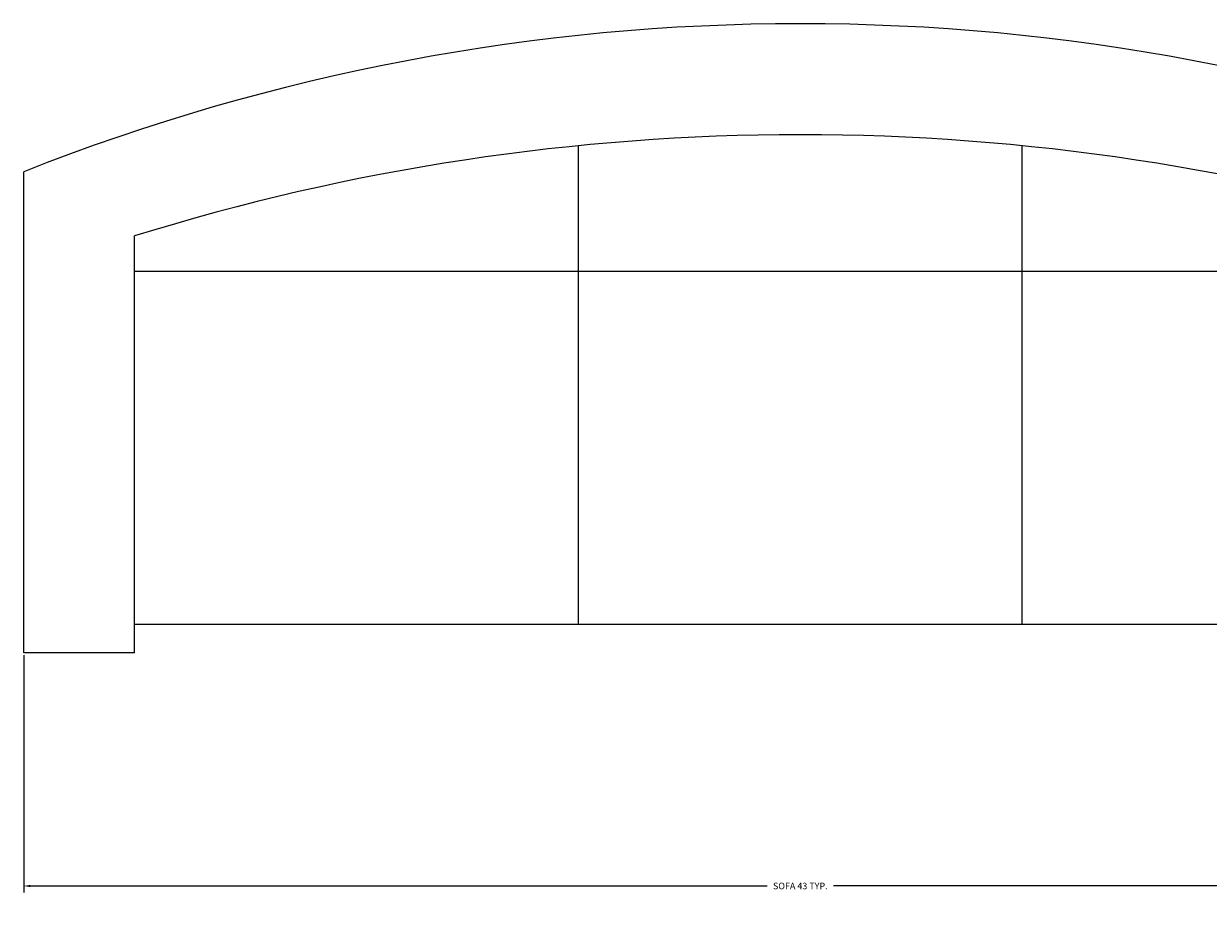
# Model space of a CAD drawing. Units: feet. Extents: x 2219 to 3039, y 1768 to 2369.
# Tile 9 of 16: x 2731 to 2764, y 2292 to 2316. Entities that reach past the tile are written whole.
import ezdxf

# ---------------------------------------------------------------- set-up
doc = ezdxf.new("R2010")
doc.units = ezdxf.units.FT
doc.layers.add('A-ANNO-DIMS', color=2, linetype='Continuous', lineweight=18)
doc.layers.add('A-FURN', color=8, linetype='Continuous', lineweight=18)
doc.styles.get("Standard").update_dxf_attribs({"font": 'arial.ttf'})
doc.dimstyles.get("Standard").update_dxf_attribs({"dimtxt": 0.18, "dimasz": 0.18, "dimexe": 0.18, "dimexo": 0.0625, "dimgap": 0.09, "dimtad": 0, "dimtih": 1, "dimtoh": 1, "dimdec": 4, "dimzin": 0, "dimdsep": 46, "dimtxsty": 'Standard', "dimcen": 0.09, "dimadec": 0, "dimazin": 0, "dimtfac": 1, "dimtdec": 4, "dimtofl": 0, "dimtmove": 0, "dimatfit": 3, "dimfxl": 1, "dimtolj": 1, "dimtzin": 0, "dimarcsym": 0})

# ---------------------------------------------------------------- blocks, each defined once
blk = doc.blocks.new('Sofa - Roundback 7 ft.')
for p, q in [((-12.00002, -32.4421), (-12.00003, -6.5971)), ((11.99997, -32.4421), (11.99998, -6.5971)), ((-36.000027, -34), (-36.000027, -11.4696)), ((-35.999844, -13.3819), (35.9998, -13.3819)), ((-36.000027, -32.4421), (35.99998, -32.4421))]:
    blk.add_line(p, q)
blk.add_lwpolyline([(-36.000027, -34), (-42.000027, -34), (-42.000027, -8)])
for centre, radius, start, end in [((0, -114.25), 114.25, 68.43141, 111.5686), ((-0.00001, -127.1968), 121.1968, 72.72033, 107.2797)]:
    blk.add_arc(centre, radius, start, end)
blk = doc.blocks.new('*D24')
at = {"layer": 'A-ANNO-DIMS', "color": 0, "lineweight": -2, "transparency": 16777216}
for p, q in [((2731.366, 2298.238), (2731.366, 2291.74)), ((2773.903, 2298.238), (2773.903, 2291.74)), ((2731.546, 2291.92), (2751.73, 2291.92)), ((2773.723, 2291.92), (2753.54, 2291.92))]:
    blk.add_line(p, q, dxfattribs=at)
at = {"layer": 'A-ANNO-DIMS', "color": 0, "transparency": 16777216}
for points in [[(2731.546, 2291.95), (2731.546, 2291.89), (2731.366, 2291.92)], [(2773.723, 2291.95), (2773.723, 2291.89), (2773.903, 2291.92)]]:
    blk.add_solid(points, dxfattribs=at)
at = {"layer": 'Defpoints', "color": 0, "transparency": 16777216}
for p in [(2731.366, 2298.3), (2773.903, 2298.3), (2773.903, 2291.92)]:
    blk.add_point(p, dxfattribs=at)
at = {"layer": 'A-ANNO-DIMS', "color": 0, "transparency": 16777216, "insert": (2752.635, 2291.92), "char_height": 0.18, "attachment_point": 5}
blk.add_mtext('\\A1;SOFA 43 TYP.', dxfattribs=at)

msp = doc.modelspace()

# ---------------------------------------------------------------- block references
at = {"layer": 'A-FURN', "xscale": 0.5063942958922181, "yscale": 0.5063942958922181, "zscale": 0.5063942958922181}
msp.add_blockref('Sofa - Roundback 7 ft.', (2752.635, 2315.518), dxfattribs=at)

# ---------------------------------------------------------------- dimensions: what is measured, and where the dimension line sits
at = {"layer": 'A-ANNO-DIMS'}
dim = msp.add_linear_dim(base=(2773.903, 2291.92), p1=(2731.366, 2298.3), p2=(2773.903, 2298.3), text='SOFA <> TYP.', dimstyle='Standard', override={"dimdec": 0, "dimlfac": 1, "dimrnd": 0, "dimzin": 0, "dimdsep": 46, "dimlunit": 2}, dxfattribs=at)
dim.commit()
dim.dimension.update_dxf_attribs({"geometry": '*D24', "text_midpoint": (2752.635, 2291.92)})

doc.saveas('drawing.dxf')
